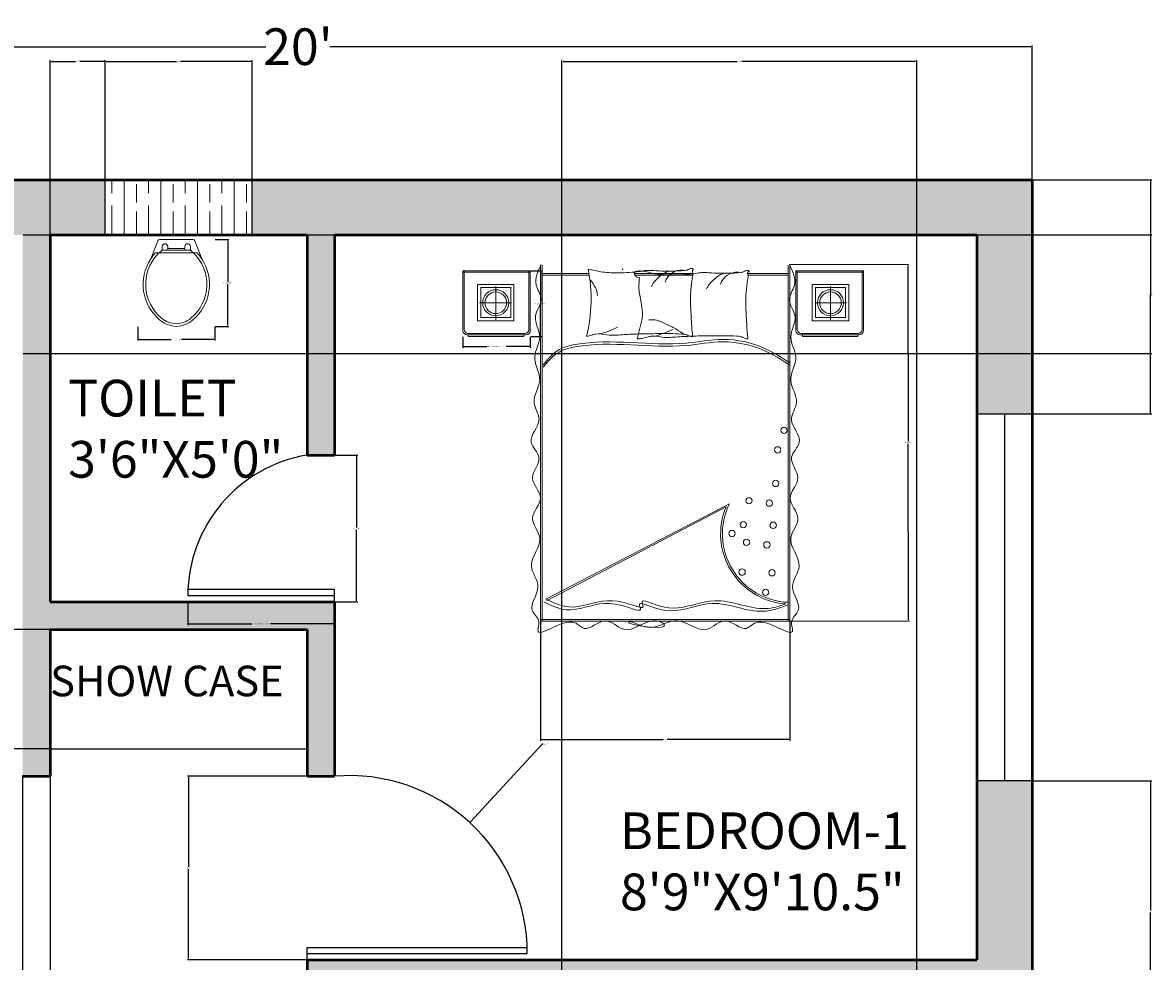
# Model space of a CAD drawing. Units: inches. Extents: x -2 to 282, y -370 to 35.
# Tile 5 of 5: x 97 to 282, y -119 to 35. Entities that reach past the tile are written whole.
import ezdxf

# ---------------------------------------------------------------- set-up
doc = ezdxf.new("R2010")
doc.units = ezdxf.units.IN
doc.header["$MEASUREMENT"] = 0
for name, color, linetype, lineweight in [('A-ANNO-DIMS', 2, 'Continuous', 18), ('A-ANNO-TEXT', 7, 'Continuous', 18), ('A-AREA-IDEN', 7, 'Continuous', 25), ('A-DOOR', 3, 'Continuous', 25), ('A-FLOR-CASE', 8, 'Continuous', 25), ('A-FLOR-FIXT', 9, 'Continuous', 18), ('A-FURN', 8, 'Continuous', 18), ('A-GLAZ', 4, 'Continuous', 25), ('A-GLAZ-PATT', 9, 'Continuous', 13), ('A-WALL', 7, 'Continuous', 50), ('A-WALL-PATT', 252, 'Continuous', 13)]:
    doc.layers.add(name, color=color, linetype=linetype, lineweight=lineweight)
doc.styles.get("Standard").update_dxf_attribs({"font": 'arial.ttf'})
doc.dimstyles.get("Standard").update_dxf_attribs({"dimtxt": 0.18, "dimasz": 0.18, "dimexe": 0.18, "dimexo": 0.0625, "dimgap": 0.09, "dimtad": 0, "dimtih": 1, "dimtoh": 1, "dimdec": 0, "dimzin": 0, "dimdsep": 46, "dimlunit": 3, "dimtxsty": 'Standard', "dimcen": 0.09, "dimadec": 0, "dimazin": 0, "dimtfac": 1, "dimtdec": 0, "dimtofl": 0, "dimtmove": 0, "dimatfit": 3, "dimfxl": 1, "dimtolj": 1, "dimtzin": 0, "dimarcsym": 0})

# ---------------------------------------------------------------- blocks, each defined once
blk = doc.blocks.new('*D3')
at = {"layer": 'A-ANNO-DIMS', "color": 0, "lineweight": -2, "transparency": 16777216}
for p, q in [((22.41, 9.25), (22.41, 31.14)), ((22.59, 30.96), (137.18, 30.96)), ((262.23, 30.96), (147.65, 30.96)), ((262.41, 9.25), (262.41, 31.14))]:
    blk.add_line(p, q, dxfattribs=at)
at = {"layer": 'A-ANNO-DIMS', "color": 0, "transparency": 16777216}
for points in [[(22.59, 30.99), (22.59, 30.93), (22.41, 30.96)], [(262.23, 30.99), (262.23, 30.93), (262.41, 30.96)]]:
    blk.add_solid(points, dxfattribs=at)
at = {"layer": 'Defpoints', "color": 0, "transparency": 16777216}
for p in [(262.41, 30.96), (22.41, 9.19), (262.41, 9.19)]:
    blk.add_point(p, dxfattribs=at)
at = {"layer": 'A-ANNO-DIMS', "color": 0, "transparency": 16777216, "insert": (142.41, 30.96), "char_height": 6, "attachment_point": 5}
blk.add_mtext("\\A1;20'", dxfattribs=at)
blk = doc.blocks.new('WINDOW-60IN')
for p, q in [((0, 0), (0, 60)), ((0, 60), (9, 60)), ((4.5, 60), (4.5, 0)), ((9, 60), (9, 0)), ((9, 0), (0, 0))]:
    blk.add_line(p, q)
blk = doc.blocks.new('DOOR-SWING-24IN')
for p, q in [((24, 2), (0, 2)), ((24, 0), (24, 2)), ((24, 1), (0, 1))]:
    blk.add_line(p, q)
blk.add_arc((23.32, 1), 23.31, 99.4157, 180)
blk = doc.blocks.new('WC-PLAN')
for p, q in [((2.03, 12.04), (2.63, 12.04)), ((2.63, 12.04), (5.42, 12.04)), ((8.21, 12.04), (5.42, 12.04)), ((8.21, 12.04), (8.81, 12.04))]:
    blk.add_line(p, q)
for points in [[(5.42, 14.19), (2.71, 14.19, 0.31031), (2.38, 13.97), (1.26, 11.07, 0.209071)], [(3.12, 12.47), (3.12, 13.07, -1), (4.02, 13.07), (4.02, 12.76)], [(5.42, 14.19), (8.13, 14.19, -0.31031), (8.46, 13.97), (9.58, 11.07, -0.209071)], [(7.72, 12.47), (7.72, 13.07, 1), (6.82, 13.07), (6.82, 12.76)], [(2.34, 11.76, 0.431639), (3.02, 1.35, 0.162618), (5.42, 0.42, 0.470877)], [(2.03, 12.04, 0.040937), (1.26, 11.07, 0.163732)], [(2.63, 12.04, 0.014165), (2.34, 11.76, 0.162618)], [(3.12, 12.47, 0.022712), (2.63, 12.04, 0.162618)], [(5.42, 12.47), (3.12, 12.47, 0.022712)], [(5.42, 12.47), (7.72, 12.47, -0.476108)], [(8.21, 12.04, -0.448546), (7.82, 1.35, -0.162618), (5.42, 0.42, -0.470877)], [(7.72, 12.47, -0.022712), (8.21, 12.04, -0.162618)], [(8.81, 12.04, -0.040937), (9.58, 11.07, -0.163732)], [(1.26, 11.07, 0.383919), (2.75, 1.02, 0.163732), (5.42, 0, 0.359733)], [(9.58, 11.07, -0.383919), (8.09, 1.02, -0.163732), (5.42, 0, -0.359733)]]:
    blk.add_lwpolyline(points, format="xyb")
for points in [[(6.82, 12.76), (4.02, 12.76)], [(4.02, 12.76), (4.02, 12.47)], [(6.82, 12.76), (6.82, 12.47)]]:
    blk.add_lwpolyline(points)
blk = doc.blocks.new('BEDSIDE-TABLE')
for p, q in [((0, 0.94), (0, 10.72)), ((0, 10.72), (11.02, 10.72)), ((0, 10.5), (11.02, 10.5)), ((0.22, 1.16), (0.22, 10.72)), ((10.8, 10.72), (10.8, 1.16)), ((11.02, 10.72), (11.02, 0.94)), ((2.39, 8.51), (2.39, 2.55)), ((8.35, 8.51), (2.39, 8.51)), ((2.92, 7.98), (2.92, 3.08)), ((7.82, 7.98), (2.92, 7.98)), ((5.37, 2.73), (5.37, 8.22)), ((7.82, 7.98), (7.82, 3.08)), ((8.35, 8.51), (8.35, 2.55)), ((7.94, 5.51), (2.73, 5.51)), ((8.35, 2.55), (2.39, 2.55)), ((7.82, 3.08), (2.92, 3.08)), ((10.37, 0.28), (0.66, 0.28)), ((10.15, 0.5), (0.87, 0.5))]:
    blk.add_line(p, q)
blk.add_lwpolyline([(9.94, 0.26), (0.88, 0.26), (0.88, 0), (9.94, 0)], close=True)
for radius in [2.13, 1.77]:
    blk.add_circle((5.37, 5.51), radius)
for centre, start, end in [((0.66, 0.94), 180, 270), ((0.87, 1.16), 180, 270), ((10.15, 1.16), 270, 0), ((10.37, 0.94), 270, 0)]:
    blk.add_arc(centre, 0.655, start, end)
blk = doc.blocks.new('*D13')
at = {"layer": 'A-ANNO-DIMS', "color": 0, "lineweight": -2, "transparency": 16777216}
for p, q in [((169.38, -16.48), (169.38, -18.25)), ((180.4, -16.48), (180.4, -18.25)), ((169.56, -18.07), (173.34, -18.07)), ((180.22, -18.07), (176.45, -18.07))]:
    blk.add_line(p, q, dxfattribs=at)
at = {"layer": 'A-ANNO-DIMS', "color": 0, "transparency": 16777216}
for points in [[(169.56, -18.04), (169.56, -18.1), (169.38, -18.07)], [(180.22, -18.04), (180.22, -18.1), (180.4, -18.07)]]:
    blk.add_solid(points, dxfattribs=at)
at = {"layer": 'Defpoints', "color": 0, "transparency": 16777216}
for p in [(169.38, -16.41), (180.4, -16.41), (180.4, -18.07)]:
    blk.add_point(p, dxfattribs=at)
at = {"layer": 'A-ANNO-DIMS', "color": 0, "transparency": 16777216, "insert": (174.89, -18.07), "char_height": 0.18, "attachment_point": 5}
blk.add_mtext('\\A1;NIGHTSTAND 0\'-11" TYP.', dxfattribs=at)
blk = doc.blocks.new('*D14')
at = {"layer": 'A-ANNO-DIMS', "color": 0, "lineweight": -2, "transparency": 16777216}
for p, q in [((180.46, -5.69), (182.24, -5.69)), ((182.06, -5.87), (182.06, -10.87)), ((182.06, -16.23), (182.06, -11.23)), ((180.46, -16.41), (182.24, -16.41))]:
    blk.add_line(p, q, dxfattribs=at)
at = {"layer": 'A-ANNO-DIMS', "color": 0, "transparency": 16777216}
for points in [[(182.03, -5.87), (182.09, -5.87), (182.06, -5.69)], [(182.03, -16.23), (182.09, -16.23), (182.06, -16.41)]]:
    blk.add_solid(points, dxfattribs=at)
at = {"layer": 'Defpoints', "color": 0, "transparency": 16777216}
for p in [(180.4, -5.69), (182.06, -5.69), (180.4, -16.41)]:
    blk.add_point(p, dxfattribs=at)
at = {"layer": 'A-ANNO-DIMS', "color": 0, "transparency": 16777216, "insert": (182.06, -11.05), "char_height": 0.18, "attachment_point": 5}
blk.add_mtext('\\A1;0\'-10 1/2" TYP.', dxfattribs=at)
blk = doc.blocks.new('*D17')
at = {"layer": 'A-ANNO-DIMS', "color": 0, "lineweight": -2, "transparency": 16777216}
for p, q in [((124.41, -59.87), (124.41, -63.59)), ((148.41, -59.87), (148.41, -63.59)), ((124.59, -63.41), (134.89, -63.41)), ((148.23, -63.41), (137.94, -63.41))]:
    blk.add_line(p, q, dxfattribs=at)
at = {"layer": 'A-ANNO-DIMS', "color": 0, "transparency": 16777216}
for points in [[(124.59, -63.38), (124.59, -63.44), (124.41, -63.41)], [(148.23, -63.38), (148.23, -63.44), (148.41, -63.41)]]:
    blk.add_solid(points, dxfattribs=at)
at = {"layer": 'Defpoints', "color": 0, "transparency": 16777216}
for p in [(124.41, -59.81), (148.41, -59.81), (148.41, -63.41)]:
    blk.add_point(p, dxfattribs=at)
at = {"layer": 'A-ANNO-DIMS', "color": 0, "transparency": 16777216, "insert": (136.41, -63.41), "char_height": 0.18, "attachment_point": 5}
blk.add_mtext('\\A1;TOILET DOOR 2\'-0" TYP.', dxfattribs=at)
blk = doc.blocks.new('*D18')
at = {"layer": 'A-ANNO-DIMS', "color": 0, "lineweight": -2, "transparency": 16777216}
for p, q in [((148.48, -35.81), (152.19, -35.81)), ((152.01, -35.99), (152.01, -47.63)), ((152.01, -59.63), (152.01, -47.99)), ((148.48, -59.81), (152.19, -59.81))]:
    blk.add_line(p, q, dxfattribs=at)
at = {"layer": 'A-ANNO-DIMS', "color": 0, "transparency": 16777216}
for points in [[(151.98, -35.99), (152.04, -35.99), (152.01, -35.81)], [(151.98, -59.63), (152.04, -59.63), (152.01, -59.81)]]:
    blk.add_solid(points, dxfattribs=at)
at = {"layer": 'Defpoints', "color": 0, "transparency": 16777216}
for p in [(148.41, -35.81), (152.01, -35.81), (148.41, -59.81)]:
    blk.add_point(p, dxfattribs=at)
at = {"layer": 'A-ANNO-DIMS', "color": 0, "transparency": 16777216, "insert": (152.01, -47.81), "char_height": 0.18, "attachment_point": 5}
blk.add_mtext('\\A1;2\'-0" TYP.', dxfattribs=at)
blk = doc.blocks.new('*D19')
at = {"layer": 'A-ANNO-DIMS', "color": 0, "lineweight": -2, "transparency": 16777216}
for p, q in [((128.9, -0.58), (131.14, -0.58)), ((130.96, -0.76), (130.96, -7.49)), ((130.96, -14.59), (130.96, -7.86)), ((128.9, -14.77), (131.14, -14.77))]:
    blk.add_line(p, q, dxfattribs=at)
at = {"layer": 'A-ANNO-DIMS', "color": 0, "transparency": 16777216}
for points in [[(130.93, -0.76), (130.99, -0.76), (130.96, -0.58)], [(130.93, -14.59), (130.99, -14.59), (130.96, -14.77)]]:
    blk.add_solid(points, dxfattribs=at)
at = {"layer": 'Defpoints', "color": 0, "transparency": 16777216}
for p in [(128.84, -0.58), (130.96, -0.58), (128.84, -14.77)]:
    blk.add_point(p, dxfattribs=at)
at = {"layer": 'A-ANNO-DIMS', "color": 0, "transparency": 16777216, "insert": (130.96, -7.67), "char_height": 0.18, "attachment_point": 5}
blk.add_mtext('\\A1;WC 1\'-2" TYP.', dxfattribs=at)
blk = doc.blocks.new('*D20')
at = {"layer": 'A-ANNO-DIMS', "color": 0, "lineweight": -2, "transparency": 16777216}
for p, q in [((116.23, -14.83), (116.23, -17.08)), ((128.84, -14.83), (128.84, -17.08)), ((116.41, -16.9), (121.69, -16.9)), ((128.66, -16.9), (123.37, -16.9))]:
    blk.add_line(p, q, dxfattribs=at)
at = {"layer": 'A-ANNO-DIMS', "color": 0, "transparency": 16777216}
for points in [[(116.41, -16.87), (116.41, -16.93), (116.23, -16.9)], [(128.66, -16.87), (128.66, -16.93), (128.84, -16.9)]]:
    blk.add_solid(points, dxfattribs=at)
at = {"layer": 'Defpoints', "color": 0, "transparency": 16777216}
for p in [(116.23, -14.77), (128.84, -14.77), (128.84, -16.9)]:
    blk.add_point(p, dxfattribs=at)
at = {"layer": 'A-ANNO-DIMS', "color": 0, "transparency": 16777216, "insert": (122.53, -16.9), "char_height": 0.18, "attachment_point": 5}
blk.add_mtext('\\A1;1\'-0 1/2" TYP.', dxfattribs=at)
blk = doc.blocks.new('*D25')
at = {"layer": 'A-ANNO-DIMS', "color": 0, "lineweight": -2, "transparency": 16777216}
for p, q in [((262.48, 9.19), (281.97, 9.19)), ((281.79, 9.01), (281.79, -9.75)), ((281.79, -28.88), (281.79, -10.12)), ((262.48, -29.06), (281.97, -29.06))]:
    blk.add_line(p, q, dxfattribs=at)
at = {"layer": 'A-ANNO-DIMS', "color": 0, "transparency": 16777216}
for points in [[(281.76, 9.01), (281.82, 9.01), (281.79, 9.19)], [(281.76, -28.88), (281.82, -28.88), (281.79, -29.06)]]:
    blk.add_solid(points, dxfattribs=at)
at = {"layer": 'Defpoints', "color": 0, "transparency": 16777216}
for p in [(262.41, 9.19), (262.41, -29.06), (281.79, -29.06)]:
    blk.add_point(p, dxfattribs=at)
at = {"layer": 'A-ANNO-DIMS', "color": 0, "transparency": 16777216, "insert": (281.79, -9.94), "char_height": 0.18, "attachment_point": 5}
blk.add_mtext('\\A1;3\'-2 1/2"', dxfattribs=at)
blk = doc.blocks.new('*D26')
at = {"layer": 'A-ANNO-DIMS', "color": 0, "lineweight": -2, "transparency": 16777216}
for p, q in [((262.48, -89.06), (281.97, -89.06)), ((281.79, -89.24), (281.79, -110.25)), ((281.79, -131.63), (281.79, -110.62)), ((262.48, -131.81), (281.97, -131.81))]:
    blk.add_line(p, q, dxfattribs=at)
at = {"layer": 'A-ANNO-DIMS', "color": 0, "transparency": 16777216}
for points in [[(281.76, -89.24), (281.82, -89.24), (281.79, -89.06)], [(281.76, -131.63), (281.82, -131.63), (281.79, -131.81)]]:
    blk.add_solid(points, dxfattribs=at)
at = {"layer": 'Defpoints', "color": 0, "transparency": 16777216}
for p in [(262.41, -89.06), (262.41, -131.81), (281.79, -131.81)]:
    blk.add_point(p, dxfattribs=at)
at = {"layer": 'A-ANNO-DIMS', "color": 0, "transparency": 16777216, "insert": (281.79, -110.44), "char_height": 0.18, "attachment_point": 5}
blk.add_mtext('\\A1;3\'-7"', dxfattribs=at)
blk = doc.blocks.new('*D33')
at = {"layer": 'A-ANNO-DIMS', "color": 0, "lineweight": -2, "transparency": 16777216}
for p, q in [((101.91, 0.25), (101.91, 28.74)), ((102.09, 28.56), (106.08, 28.56)), ((110.73, 28.56), (106.74, 28.56)), ((110.91, 0.25), (110.91, 28.74))]:
    blk.add_line(p, q, dxfattribs=at)
at = {"layer": 'A-ANNO-DIMS', "color": 0, "transparency": 16777216}
for points in [[(102.09, 28.59), (102.09, 28.53), (101.91, 28.56)], [(110.73, 28.59), (110.73, 28.53), (110.91, 28.56)]]:
    blk.add_solid(points, dxfattribs=at)
at = {"layer": 'Defpoints', "color": 0, "transparency": 16777216}
for p in [(110.91, 28.56), (101.91, 0.19), (110.91, 0.19)]:
    blk.add_point(p, dxfattribs=at)
at = {"layer": 'A-ANNO-DIMS', "color": 0, "transparency": 16777216, "insert": (106.41, 28.56), "char_height": 0.18, "attachment_point": 5}
blk.add_mtext('\\A1;0\'-9"', dxfattribs=at)
blk = doc.blocks.new('*D34')
at = {"layer": 'A-ANNO-DIMS', "color": 0, "lineweight": -2, "transparency": 16777216}
for p, q in [((110.91, 0.25), (110.91, 28.74)), ((111.09, 28.56), (122.58, 28.56)), ((134.73, 28.56), (123.24, 28.56)), ((134.91, 0.25), (134.91, 28.74))]:
    blk.add_line(p, q, dxfattribs=at)
at = {"layer": 'A-ANNO-DIMS', "color": 0, "transparency": 16777216}
for points in [[(111.09, 28.59), (111.09, 28.53), (110.91, 28.56)], [(134.73, 28.59), (134.73, 28.53), (134.91, 28.56)]]:
    blk.add_solid(points, dxfattribs=at)
at = {"layer": 'Defpoints', "color": 0, "transparency": 16777216}
for p in [(134.91, 28.56), (110.91, 0.19), (134.91, 0.19)]:
    blk.add_point(p, dxfattribs=at)
at = {"layer": 'A-ANNO-DIMS', "color": 0, "transparency": 16777216, "insert": (122.91, 28.56), "char_height": 0.18, "attachment_point": 5}
blk.add_mtext('\\A1;2\'-0"', dxfattribs=at)
blk = doc.blocks.new('*D39')
at = {"layer": 'A-ANNO-DIMS', "color": 0, "lineweight": -2, "transparency": 16777216}
for p, q in [((64.41, -88.37), (64.41, -370.37)), ((97.41, -88.37), (97.41, -370.37)), ((64.59, -370.19), (80.58, -370.19)), ((97.23, -370.19), (81.24, -370.19))]:
    blk.add_line(p, q, dxfattribs=at)
at = {"layer": 'A-ANNO-DIMS', "color": 0, "transparency": 16777216}
for points in [[(64.59, -370.16), (64.59, -370.22), (64.41, -370.19)], [(97.23, -370.16), (97.23, -370.22), (97.41, -370.19)]]:
    blk.add_solid(points, dxfattribs=at)
at = {"layer": 'Defpoints', "color": 0, "transparency": 16777216}
for p in [(64.41, -88.31), (97.41, -88.31), (97.41, -370.19)]:
    blk.add_point(p, dxfattribs=at)
at = {"layer": 'A-ANNO-DIMS', "color": 0, "transparency": 16777216, "insert": (80.91, -370.19), "char_height": 0.18, "attachment_point": 5}
blk.add_mtext('\\A1;2\'-9"', dxfattribs=at)
blk = doc.blocks.new('*D43')
at = {"layer": 'A-ANNO-DIMS', "color": 0, "lineweight": -2, "transparency": 16777216}
for p, q in [((97.48, 0.19), (281.97, 0.19)), ((281.79, 0.01), (281.79, -9.33)), ((281.79, -19.03), (281.79, -9.69)), ((97.48, -19.21), (281.97, -19.21))]:
    blk.add_line(p, q, dxfattribs=at)
at = {"layer": 'A-ANNO-DIMS', "color": 0, "transparency": 16777216}
for points in [[(281.76, 0.01), (281.82, 0.01), (281.79, 0.19)], [(281.76, -19.03), (281.82, -19.03), (281.79, -19.21)]]:
    blk.add_solid(points, dxfattribs=at)
at = {"layer": 'Defpoints', "color": 0, "transparency": 16777216}
for p in [(97.41, 0.19), (97.41, -19.21), (281.79, -19.21)]:
    blk.add_point(p, dxfattribs=at)
at = {"layer": 'A-ANNO-DIMS', "color": 0, "transparency": 16777216, "insert": (281.79, -9.51), "char_height": 0.18, "attachment_point": 5}
blk.add_mtext('\\A1;1\'-7 1/2"', dxfattribs=at)
blk = doc.blocks.new('*D45')
at = {"layer": 'A-ANNO-DIMS', "color": 0, "lineweight": -2, "transparency": 16777216}
for p, q in [((101.85, -64.31), (2.86, -64.31)), ((3.04, -64.49), (3.04, -73.88)), ((3.04, -83.63), (3.04, -74.24)), ((101.85, -83.81), (2.86, -83.81))]:
    blk.add_line(p, q, dxfattribs=at)
at = {"layer": 'A-ANNO-DIMS', "color": 0, "transparency": 16777216}
for points in [[(3.01, -64.49), (3.07, -64.49), (3.04, -64.31)], [(3.01, -83.63), (3.07, -83.63), (3.04, -83.81)]]:
    blk.add_solid(points, dxfattribs=at)
at = {"layer": 'Defpoints', "color": 0, "transparency": 16777216}
for p in [(101.91, -64.31), (3.04, -83.81), (101.91, -83.81)]:
    blk.add_point(p, dxfattribs=at)
at = {"layer": 'A-ANNO-DIMS', "color": 0, "transparency": 16777216, "insert": (3.04, -74.06), "char_height": 0.18, "attachment_point": 5}
blk.add_mtext('\\A1;1\'-7 1/2"', dxfattribs=at)
blk = doc.blocks.new('*D46')
at = {"layer": 'A-ANNO-DIMS', "color": 0, "lineweight": -2, "transparency": 16777216}
for p, q in [((97.41, -88.37), (97.41, -370.37)), ((101.91, -88.37), (101.91, -370.37)), ((97.59, -370.19), (99.12, -370.19)), ((101.73, -370.19), (100.2, -370.19))]:
    blk.add_line(p, q, dxfattribs=at)
at = {"layer": 'A-ANNO-DIMS', "color": 0, "transparency": 16777216}
for points in [[(97.59, -370.16), (97.59, -370.22), (97.41, -370.19)], [(101.73, -370.16), (101.73, -370.22), (101.91, -370.19)]]:
    blk.add_solid(points, dxfattribs=at)
at = {"layer": 'Defpoints', "color": 0, "transparency": 16777216}
for p in [(97.41, -88.31), (101.91, -88.31), (101.91, -370.19)]:
    blk.add_point(p, dxfattribs=at)
at = {"layer": 'A-ANNO-DIMS', "color": 0, "transparency": 16777216, "insert": (99.66, -370.19), "char_height": 0.18, "attachment_point": 5}
blk.add_mtext('\\A1;0\'-4 1/2"', dxfattribs=at)
blk = doc.blocks.new('*D52')
at = {"layer": 'A-ANNO-DIMS', "color": 0, "lineweight": -2, "transparency": 16777216}
for p, q in [((185.58, -222.52), (185.58, 28.74)), ((185.76, 28.56), (214.16, 28.56)), ((243.38, 28.56), (214.97, 28.56)), ((243.56, -222.52), (243.56, 28.74))]:
    blk.add_line(p, q, dxfattribs=at)
at = {"layer": 'A-ANNO-DIMS', "color": 0, "transparency": 16777216}
for points in [[(185.76, 28.59), (185.76, 28.53), (185.58, 28.56)], [(243.38, 28.59), (243.38, 28.53), (243.56, 28.56)]]:
    blk.add_solid(points, dxfattribs=at)
at = {"layer": 'Defpoints', "color": 0, "transparency": 16777216}
for p in [(243.56, 28.56), (185.58, -222.58), (243.56, -222.58)]:
    blk.add_point(p, dxfattribs=at)
at = {"layer": 'A-ANNO-DIMS', "color": 0, "transparency": 16777216, "insert": (214.57, 28.56), "char_height": 0.18, "attachment_point": 5}
blk.add_mtext('\\A1;4\'-10"', dxfattribs=at)
blk = doc.blocks.new('*D54')
at = {"layer": 'A-ANNO-DIMS', "color": 0, "lineweight": -2, "transparency": 16777216}
for p, q in [((182.07, -63.02), (182.07, -82.51)), ((222.85, -63.02), (222.85, -82.51)), ((182.25, -82.33), (202.13, -82.33)), ((222.67, -82.33), (202.79, -82.33))]:
    blk.add_line(p, q, dxfattribs=at)
at = {"layer": 'A-ANNO-DIMS', "color": 0, "transparency": 16777216}
for points in [[(182.25, -82.3), (182.25, -82.36), (182.07, -82.33)], [(222.67, -82.3), (222.67, -82.36), (222.85, -82.33)]]:
    blk.add_solid(points, dxfattribs=at)
at = {"layer": 'Defpoints', "color": 0, "transparency": 16777216}
for p in [(182.07, -62.96), (222.85, -62.96), (182.07, -82.33)]:
    blk.add_point(p, dxfattribs=at)
at = {"layer": 'A-ANNO-DIMS', "color": 0, "transparency": 16777216, "insert": (202.46, -82.33), "char_height": 0.18, "attachment_point": 5}
blk.add_mtext('\\A1;3\'-5"', dxfattribs=at)
blk = doc.blocks.new('*D55')
at = {"layer": 'A-ANNO-DIMS', "color": 0, "lineweight": -2, "transparency": 16777216}
for p, q in [((222.81, -4.64), (242.3, -4.61)), ((242.12, -4.79), (242.18, -33.58)), ((242.23, -62.74), (242.18, -33.95)), ((222.91, -62.96), (242.41, -62.92))]:
    blk.add_line(p, q, dxfattribs=at)
at = {"layer": 'A-ANNO-DIMS', "color": 0, "transparency": 16777216}
for points in [[(242.15, -4.79), (242.09, -4.79), (242.12, -4.61)], [(242.26, -62.74), (242.2, -62.74), (242.23, -62.92)]]:
    blk.add_solid(points, dxfattribs=at)
at = {"layer": 'Defpoints', "color": 0, "transparency": 16777216}
for p in [(222.75, -4.64), (222.85, -62.96), (242.23, -62.92)]:
    blk.add_point(p, dxfattribs=at)
at = {"layer": 'A-ANNO-DIMS', "color": 0, "transparency": 16777216, "insert": (242.18, -33.77), "char_height": 0.18, "attachment_point": 5}
blk.add_mtext('\\A1;4\'-10 1/2"', dxfattribs=at)
blk = doc.blocks.new('*D58')
at = {"layer": 'A-ANNO-DIMS', "color": 0, "lineweight": -2, "transparency": 16777216}
for p, q in [((143.85, -88.31), (124.36, -88.31)), ((124.54, -88.49), (124.54, -103.13)), ((124.54, -118.13), (124.54, -103.49)), ((143.85, -118.31), (124.36, -118.31))]:
    blk.add_line(p, q, dxfattribs=at)
at = {"layer": 'A-ANNO-DIMS', "color": 0, "transparency": 16777216}
for points in [[(124.51, -88.49), (124.57, -88.49), (124.54, -88.31)], [(124.51, -118.13), (124.57, -118.13), (124.54, -118.31)]]:
    blk.add_solid(points, dxfattribs=at)
at = {"layer": 'Defpoints', "color": 0, "transparency": 16777216}
for p in [(124.54, -88.31), (143.91, -88.31), (143.91, -118.31)]:
    blk.add_point(p, dxfattribs=at)
at = {"layer": 'A-ANNO-DIMS', "color": 0, "transparency": 16777216, "insert": (124.54, -103.31), "char_height": 0.18, "attachment_point": 5}
blk.add_mtext('\\A1;2\'-6"', dxfattribs=at)
blk = doc.blocks.new('*D60')
at = {"layer": 'A-ANNO-DIMS', "color": 0, "lineweight": -2, "transparency": 16777216}
for p, q in [((182.35, -83.06), (170.65, -95.77)), ((182.53, -83.06), (182.35, -83.06)), ((150.72, -117.31), (150.9, -117.31)), ((150.81, -117.4), (150.81, -117.22))]:
    blk.add_line(p, q, dxfattribs=at)
at = {"layer": 'A-ANNO-DIMS', "color": 0, "transparency": 16777216}
blk.add_solid([(170.62, -95.75), (170.67, -95.79), (170.52, -95.9)], dxfattribs=at)
at = {"layer": 'Defpoints', "color": 0, "transparency": 16777216}
for p in [(170.52, -95.9), (150.81, -117.31)]:
    blk.add_point(p, dxfattribs=at)
at = {"layer": 'A-ANNO-DIMS', "color": 0, "transparency": 16777216, "insert": (182.94, -83.06), "char_height": 0.18, "attachment_point": 5}
blk.add_mtext('\\A1;R2\'-5"', dxfattribs=at)

msp = doc.modelspace()

# ---------------------------------------------------------------- hatches: boundary and pattern name
at = {"layer": 'A-GLAZ-PATT'}
h = msp.add_hatch(dxfattribs=at)
h.set_pattern_fill('GOST_WOOD', color=256)
h.set_pattern_definition([(90, (0, 0), (6, -4e-16), [10, -2]), (90, (2, -2), (6, -4e-16), [6, -1.5, 3, -1.5]), (90, (4, -5), (6, -4e-16), [10, -2])])
h.paths.add_polyline_path([(134.91, 9.19), (110.91, 9.19), (110.91, 0.19), (134.91, 0.19)])
h.paths.add_polyline_path([(262.41, -131.81), (253.41, -131.81), (253.41, -155.81), (262.41, -155.81)])
at = {"layer": 'A-WALL-PATT'}
h = msp.add_hatch(color=256, dxfattribs=at)
h.dxf.hatch_style = 1
h.paths.add_polyline_path([(262.41, 9.19), (134.91, 9.19), (134.91, 0.19), (143.91, 0.19), (143.91, -35.81), (148.41, -35.81), (148.41, 0.19), (253.41, 0.19), (253.41, -29.06), (262.41, -29.06)])
h.paths.add_polyline_path([(110.91, 9.19), (22.41, 9.19), (22.41, -11.81), (31.41, -11.81), (31.41, 0.19), (97.41, 0.19), (97.41, -88.31), (101.91, -88.31), (101.91, -64.31), (143.91, -64.31), (143.91, -88.31), (148.41, -88.31), (148.41, -59.81), (101.91, -59.81), (101.91, 0.19), (110.91, 0.19)])
h.paths.add_polyline_path([(31.41, -88.31), (64.41, -88.31), (64.41, -83.81), (31.41, -83.81), (31.41, -71.81), (22.41, -71.81), (22.41, -121.2), (31.41, -121.2)])
h.paths.add_polyline_path([(262.41, -89.06), (253.41, -89.06), (253.41, -118.31), (143.91, -118.31), (143.91, -122.81), (184.41, -122.81), (184.41, -164.81), (184.41, -169.31), (188.91, -169.31), (188.91, -164.81), (188.91, -122.81), (253.41, -122.81), (253.41, -131.81), (262.41, -131.81)])
h.paths.add_polyline_path([(262.41, -155.81), (253.41, -155.81), (253.41, -164.81), (212.91, -164.81), (212.91, -169.31), (253.41, -169.31), (253.41, -193.31), (262.41, -193.31)])
h.paths.add_polyline_path([(262.41, -253.31), (253.41, -253.31), (253.41, -277.31), (148.41, -277.31), (148.41, -164.81), (143.91, -164.81), (143.91, -169.31), (143.91, -281.81), (253.41, -281.81), (253.41, -341.81), (143.91, -341.81), (143.91, -350.81), (262.41, -350.81)])
h.paths.add_polyline_path([(31.41, -323.81), (22.41, -323.81), (22.41, -350.81), (95.91, -350.81), (95.91, -281.81), (107.91, -281.81), (107.91, -277.31), (67.41, -277.31), (67.41, -281.81), (91.41, -281.81), (91.41, -341.81), (31.41, -341.81)])
h.paths.add_polyline_path([(43.41, -277.31), (31.41, -277.31), (31.41, -181.2), (22.41, -181.2), (22.41, -299.81), (31.41, -299.81), (31.41, -281.81), (43.41, -281.81)])

# ---------------------------------------------------------------- linework, layer by layer
at = {"layer": 'A-DOOR'}
for p, q in [((143.91, -118.31), (143.91, -116.31)), ((143.91, -116.31), (179.91, -116.31)), ((143.91, -117.31), (179.91, -117.31))]:
    msp.add_line(p, q, dxfattribs=at)
msp.add_arc((150.81, -117.31), 29.1, 0, 94.7325, dxfattribs=at)
at = {"layer": 'A-FLOR-CASE'}
msp.add_line((101.91, -83.81), (143.91, -83.81), dxfattribs=at)
at = {"layer": 'A-FURN'}
for p, q in [((182.07, -4.74), (182.07, -62.96)), ((182.36, -4.74), (182.36, -62.96)), ((222.56, -4.74), (222.56, -62.96)), ((222.85, -4.74), (222.85, -62.96)), ((182.36, -6.13), (189.99, -6.13)), ((182.36, -6.42), (190.04, -6.42)), ((206.97, -6.13), (197.39, -6.13)), ((206.97, -6.42), (197.5, -6.42)), ((215.92, -6.13), (222.56, -6.13)), ((216, -6.42), (222.56, -6.42)), ((198.08, -15.91), (198.68, -13.51)), ((197.86, -16.79), (198.08, -15.91)), ((182.95, -59.35), (212.94, -43.77)), ((183.06, -59.63), (212.39, -44.28)), ((182.07, -62.67), (222.85, -62.67)), ((182.07, -62.96), (222.85, -62.96))]:
    msp.add_line(p, q, dxfattribs=at)
for centre in [(221.86, -31.75), (220.83, -34.96), (220.52, -40.45), (216.16, -43.25), (219.48, -43.66), (215.23, -47.18), (220.1, -47.28), (213.37, -48.63), (215.75, -50.08), (219.07, -50.49), (215.02, -54.95), (219.9, -55.05), (218.86, -58.26)]:
    msp.add_circle(centre, 0.518, dxfattribs=at)
for centre, radius, start, end in [((165.2, -10.28), 25.14, 345.9578, 11.1903), ((188.56, -14.18), 8.87, 74.256, 81.5628), ((195.46, -5.43), 0.0675, 258.1069, 19.564), ((195.43, -5.44), 0.0995, 19.564, 68.2117), ((205.57, -4.06), 1.57, 275.2592, 300.6513), ((206.8, -6.13), 0.841, 85.6975, 120.6513), ((206.81, -6.02), 0.731, 68.2117, 85.6975), ((207.03, -5.62), 0.125, 78.1069, 158.0096), ((187.34, -10.12), 4.07, 5.6311, 45.0976), ((192.88, 1.14), 7.05, 254.256, 262.4531), ((194.56, 13.85), 19.87, 262.4531, 270), ((194.56, 24.52), 30.53, 270, 276.0867), ((197.77, -6.13), 0.382, 101.2724, 206.5805), ((198.32, -5.85), 0.995, 206.5805, 265.5998), ((198.21, -8.33), 2.63, 90, 101.2724), ((196.17, 9.47), 15.41, 276.0867, 280.1899), ((212.47, -8.39), 14.32, 173.7676, 180), ((198.21, -10.39), 4.69, 81.5628, 90), ((199.68, -10.05), 4.44, 92.5386, 100.1899), ((197.6, -14.53), 8.87, 74.256, 81.5628), ((199.86, -14.05), 8.43, 85.1982, 92.5386), ((201.92, 0.8), 7.05, 254.256, 262.4531), ((202.69, 19.68), 25.42, 265.1982, 269.4243), ((205.67, -11.72), 6.55, 133.8115, 140.9651), ((203.6, 13.51), 19.87, 262.4531, 270), ((209.02, -15.21), 11.4, 128.3886, 133.8115), ((203.33, -8.03), 2.23, 117.2396, 128.3886), ((205.42, -12.1), 6.81, 110.8603, 117.2396), ((205.17, -8.45), 2.89, 85.7841, 161.5603), ((202.87, 37.76), 43.49, 269.4243, 271.9079), ((203.6, 24.17), 30.53, 270, 276.0867), ((203.52, 18.17), 23.89, 271.9079, 275.2592), ((233.14, -10.87), 26.58, 172.3191, 176.6313), ((212.53, -8.09), 5.77, 167.8905, 172.3191), ((205.2, 9.13), 15.41, 276.0867, 280.1899), ((207.34, -5.74), 0.454, 158.0096, 201.421), ((199.88, -5.38), 7.16, 347.8905, 351.8665), ((206.03, -6.25), 0.954, 351.8665, 21.421), ((208.71, -10.4), 4.44, 92.5386, 100.1899), ((208.89, -14.39), 8.43, 85.1982, 92.5386), ((211.72, 19.34), 25.42, 265.1982, 269.4243), ((214.7, -12.07), 6.55, 133.8115, 140.9651), ((218.06, -15.56), 11.4, 128.3886, 133.8115), ((212.36, -8.38), 2.23, 117.2396, 128.3886), ((214.46, -12.45), 6.81, 110.8603, 117.2396), ((214.21, -8.8), 2.89, 85.7841, 161.5603), ((211.91, 37.41), 43.49, 269.4243, 271.9079), ((212.56, 17.82), 23.89, 271.9079, 275.2592), ((214.6, -4.41), 1.57, 275.2592, 300.6513), ((215.83, -6.48), 0.841, 85.6975, 120.6513), ((221.56, -8.44), 5.77, 167.8905, 172.3191), ((215.84, -6.37), 0.731, 68.2117, 85.6975), ((216.37, -6.09), 0.454, 158.0096, 201.421), ((208.92, -5.72), 7.16, 347.8905, 351.8665), ((216.07, -5.96), 0.125, 78.1069, 158.0096), ((215.06, -6.6), 0.954, 351.8665, 21.421), ((216.11, -5.77), 0.0675, 258.1069, 19.564), ((216.08, -5.79), 0.0995, 19.564, 68.2117), ((204.09, -8.39), 5.94, 180, 189.6844), ((205.56, -10.58), 5.83, 151.6832, 156.9972), ((201.69, -8.49), 1.44, 140.9651, 151.6832), ((214.59, -10.92), 5.83, 151.6832, 156.9972), ((210.73, -8.84), 1.44, 140.9651, 151.6832), ((242.18, -11.22), 26.58, 172.3191, 176.6313), ((223.54, -5.07), 25.67, 189.6844, 192.1984), ((189.43, -12.45), 9.23, 8.0051, 12.1984), ((226.34, -10.47), 19.76, 176.6313, 181.6331), ((246.31, -9.9), 39.74, 181.6331, 183.055), ((235.37, -10.82), 19.76, 176.6313, 181.6331), ((179.58, -13.83), 19.18, 2.6649, 8.0051), ((602.96, 9.14), 396.89, 183.055, 183.5049), ((255.35, -10.25), 39.74, 181.6331, 183.055), ((611.99, 8.79), 396.89, 183.055, 183.5049), ((196.77, -13.03), 1.97, 345.9548, 2.6649), ((200.25, -21.61), 7.92, 85.9172, 93.5552), ((200.69, -15.4), 1.69, 69.3257, 85.9172), ((196.08, -27.61), 14.75, 65.6735, 69.3257), ((184.98, -52.17), 41.69, 63.5015, 65.6735), ((188.49, -9.79), 6.69, 279.4841, 287.3864), ((191.53, -19.5), 3.49, 96.4341, 107.3864), ((191.61, -20.25), 4.25, 78.4414, 96.4341), ((185.48, 4.53), 21.5, 287.1982, 295.3111), ((193.8, -9.53), 6.7, 258.4414, 272.7491), ((192.16, 24.62), 40.89, 272.7491, 274.6176), ((198.31, -51.43), 35.41, 92.6096, 94.6176), ((201.15, -113.82), 97.86, 90.9704, 92.6096), ((197.52, -10.14), 6.69, 279.4841, 287.3864), ((202.31, -182.4), 166.45, 89.7135, 90.9704), ((200.56, -19.84), 3.49, 96.4341, 107.3864), ((200.65, -20.6), 4.25, 78.4414, 96.4341), ((194.52, 4.18), 21.5, 287.1982, 295.3111), ((202.84, -9.88), 6.7, 258.4414, 272.7491), ((202.98, -49.83), 33.88, 86.426, 89.7135), ((201.2, 24.27), 40.89, 272.7491, 274.6176), ((199.52, -23), 9.1, 57.865, 63.5015), ((193.08, -33.25), 21.21, 54.1737, 57.865), ((207.34, -51.77), 35.41, 92.6096, 94.6176), ((204.82, -20.25), 4.25, 77.131, 86.426), ((210.19, -114.17), 97.86, 90.9704, 92.6096), ((205.47, -17.4), 1.32, 62.7159, 77.131), ((207.1, -14.24), 2.23, 242.7159, 253.7788), ((207.19, -13.94), 2.55, 253.7788, 262.8796), ((216.14, -14.56), 9.35, 183.5049, 189.9984), ((206.88, -16.43), 0.0385, 262.8796, 343.3022), ((206.38, -16.28), 0.563, 343.3022, 9.9984), ((211.35, -182.74), 166.45, 89.7135, 90.9704), ((212.01, -50.18), 33.88, 86.426, 89.7135), ((213.86, -20.6), 4.25, 77.131, 86.426), ((214.51, -17.74), 1.32, 62.7159, 77.131), ((216.14, -14.59), 2.23, 242.7159, 253.7788), ((225.17, -14.9), 9.35, 183.5049, 189.9984), ((215.41, -16.62), 0.563, 343.3022, 9.9984), ((197.88, -16.79), 0.0267, 165.9551, 274.0829), ((197.33, -8.96), 7.88, 274.0829, 279.4841), ((216.23, -14.29), 2.55, 253.7788, 262.8796), ((215.91, -16.77), 0.0385, 262.8796, 343.3022), ((223, -48.69), 11.49, 157.4442, 265.7493), ((223, -48.69), 11.2, 153.9063, 267.7674)]:
    msp.add_arc(centre, radius, start, end, dxfattribs=at)
for points, knots in [([(182.17, -4.64), (181.63, -5.78), (180.7, -7.72), (182.88, -10.49), (180.39, -13.27), (182.74, -16.5), (180.26, -19.94), (182.9, -23.55), (180.13, -26.96), (182.87, -30.32), (179.29, -33.44), (182.95, -36.33), (179.53, -39.58), (183.31, -42.82), (179.62, -46.1), (183.31, -49.76), (179.24, -53.61), (182.82, -57.4), (179.58, -60.87), (182.19, -62.65), (180.72, -66.65), (186.76, -61.48), (189.58, -65.14), (192.61, -61.59), (196.07, -65.77), (200.33, -61.51), (204.55, -64.87), (195.53, -63.31), (196.66, -63.02)], [0, 0, 0, 0, 119.23822, 203.934156, 305.051348, 423.414205, 538.771408, 673.601551, 801.564672, 901.488314, 1036.739405, 1131.503109, 1252.869042, 1373.114912, 1497.089457, 1612.174498, 1779.078494, 1901.133447, 2037.052147, 2110.507177, 2158.377997, 2368.992723, 2430.676444, 2554.510696, 2670.523569, 2841.287389, 2999.108306, 3118.80064, 3118.80064, 3118.80064, 3118.80064]), ([(222.75, -4.64), (223.29, -5.78), (224.22, -7.72), (222.04, -10.49), (224.53, -13.27), (222.18, -16.5), (224.66, -19.94), (222.02, -23.55), (224.79, -26.96), (222.05, -30.32), (225.63, -33.44), (221.96, -36.33), (225.38, -39.58), (221.61, -42.82), (225.3, -46.1), (221.61, -49.76), (225.68, -53.61), (222.1, -57.4), (225.34, -60.87), (222.73, -62.65), (224.2, -66.65), (218.16, -61.48), (215.34, -65.14), (212.31, -61.59), (208.85, -65.77), (204.59, -61.51), (200.37, -64.87), (197.78, -63.31), (196.66, -63.02)], [0, 0, 0, 0, 119.23822, 203.934156, 305.051348, 423.414205, 538.771408, 673.601551, 801.564672, 901.488314, 1036.739405, 1131.503109, 1252.869042, 1373.114912, 1497.089457, 1612.174498, 1779.078494, 1901.133447, 2037.052147, 2110.507177, 2158.377997, 2368.992723, 2430.676444, 2554.510696, 2670.523569, 2841.287389, 2999.108306, 3118.80064, 3118.80064, 3118.80064, 3118.80064]), ([(182.49, -21.06), (183.29, -20.11), (184.68, -18.42), (192.88, -16.42), (201.89, -18.52), (212.15, -16.46), (218.16, -17.74), (221.46, -19.84), (222.81, -20.71)], [0, 0, 0, 0, 3.612443, 6.355405, 24.536278, 30.541821, 37.462744, 42.251599, 42.251599, 42.251599, 42.251599]), ([(182.49, -21.45), (183.29, -20.49), (184.68, -18.81), (192.88, -16.81), (201.89, -18.91), (212.15, -16.85), (218.16, -18.12), (221.46, -20.23), (222.81, -21.09)], [0, 0, 0, 0, 3.612443, 6.355405, 24.536278, 30.541821, 37.462744, 42.251599, 42.251599, 42.251599, 42.251599]), ([(182.59, -59.81), (183.81, -60.4), (187, -61.94), (192.79, -58.97), (200.42, -62.56), (196.4, -58.85), (203.73, -62.27), (210.61, -58.72), (217.14, -62.24), (221.2, -60.8), (222.56, -60.29)], [0, 0, 0, 0, 134.096191, 351.943146, 593.51487, 936.925241, 1129.231545, 1368.385454, 1657.415202, 1803.02854, 1803.02854, 1803.02854, 1803.02854]), ([(183, -59.36), (184.22, -59.95), (187.42, -61.49), (193.21, -58.52), (200.83, -62.11), (196.82, -58.4), (204.14, -61.82), (211.03, -58.27), (217.27, -61.64), (221.06, -60.53), (222.15, -60.15)], [0, 0, 0, 0, 134.096191, 351.943146, 593.51487, 936.925241, 1129.231545, 1368.385454, 1657.415202, 1773.3935, 1773.3935, 1773.3935, 1773.3935])]:
    msp.add_open_spline(points, degree=3, knots=knots, dxfattribs=at)
at = {"layer": 'A-GLAZ'}
for p, q in [((110.91, 0.19), (110.91, 9.19)), ((134.91, 0.19), (134.91, 9.19))]:
    msp.add_line(p, q, dxfattribs=at)
at = {"layer": 'A-WALL'}
for p, q in [((22.41, 9.19), (262.41, 9.19)), ((262.41, 9.19), (262.41, -350.81)), ((101.91, 0.19), (101.91, -59.81)), ((101.91, 0.19), (143.91, 0.19)), ((143.91, 0.19), (143.91, -35.81)), ((148.41, 0.19), (148.41, -35.81)), ((148.41, 0.19), (253.41, 0.19)), ((253.41, 0.19), (253.41, -118.31)), ((143.91, -35.81), (148.41, -35.81)), ((101.91, -59.81), (148.41, -59.81)), ((148.41, -59.81), (148.41, -88.31)), ((101.91, -64.31), (143.91, -64.31)), ((101.91, -64.31), (101.91, -88.31)), ((143.91, -64.31), (143.91, -88.31)), ((97.41, -88.31), (101.91, -88.31)), ((143.91, -88.31), (148.41, -88.31)), ((143.91, -118.31), (253.41, -118.31)), ((143.91, -118.31), (143.91, -122.81))]:
    msp.add_line(p, q, dxfattribs=at)

# ---------------------------------------------------------------- block references
at = {"layer": 'A-DOOR'}
msp.add_blockref('DOOR-SWING-24IN', (124.41, -59.81), dxfattribs=at)
at = {"layer": 'A-FLOR-FIXT'}
msp.add_blockref('WC-PLAN', (117.11, -14.77), dxfattribs=at)
at = {"layer": 'A-FURN'}
msp.add_blockref('BEDSIDE-TABLE', (169.38, -16.41), dxfattribs=at)
at = {"layer": 'A-FURN', "extrusion": (0, 0, -1), "zscale": -1}
msp.add_blockref('BEDSIDE-TABLE', (-234.84, -16.41), dxfattribs=at)
at = {"layer": 'A-GLAZ'}
msp.add_blockref('WINDOW-60IN', (253.41, -89.06), dxfattribs=at)

# ---------------------------------------------------------------- texts
at = {"layer": 'A-ANNO-TEXT', "insert": (101.91, -70.24), "char_height": 5, "attachment_point": 1}
msp.add_mtext('SHOW CASE', dxfattribs=at)
at = {"layer": 'A-AREA-IDEN', "char_height": 6, "attachment_point": 1}
for s, insert in [('TOILET\\P3\'6"X5\'0"', (104.86, -23.5)), ('BEDROOM-1\\P8\'9"X9\'10.5"', (195.06, -94.23))]:
    msp.add_mtext(s, dxfattribs=dict(at, insert=insert))

# ---------------------------------------------------------------- dimensions: what is measured, and where the dimension line sits
at = {"layer": 'A-ANNO-DIMS'}
for base, p1, p2, override, picture, middle in [((262.41, 30.96), (22.41, 9.19), (262.41, 9.19), {"dimtxt": 6, "dimclrd": 0, "dimclre": 0, "dimclrt": 0}, '*D3', (142.41, 30.96)), ((110.91, 28.56), (101.91, 0.19), (110.91, 0.19), {"dimdec": 1, "dimlfac": 1, "dimrnd": 0, "dimzin": 1, "dimdsep": 46, "dimlunit": 4, "dimfrac": 2}, '*D33', (106.41, 28.56)), ((134.91, 28.56), (110.91, 0.19), (134.91, 0.19), {"dimdec": 1, "dimlfac": 1, "dimrnd": 0, "dimzin": 1, "dimdsep": 46, "dimlunit": 4, "dimfrac": 2}, '*D34', (122.91, 28.56)), ((243.56, 28.56), (185.58, -222.58), (243.56, -222.58), {"dimdec": 1, "dimlfac": 1, "dimrnd": 0, "dimzin": 1, "dimdsep": 46, "dimlunit": 4, "dimfrac": 2}, '*D52', (214.57, 28.56)), ((97.41, -370.19), (64.41, -88.31), (97.41, -88.31), {"dimdec": 1, "dimlfac": 1, "dimrnd": 0, "dimzin": 1, "dimdsep": 46, "dimlunit": 4, "dimfrac": 2}, '*D39', (80.91, -370.19)), ((101.91, -370.19), (97.41, -88.31), (101.91, -88.31), {"dimdec": 1, "dimlfac": 1, "dimrnd": 0, "dimzin": 1, "dimdsep": 46, "dimlunit": 4, "dimfrac": 2}, '*D46', (99.66, -370.19))]:
    dim = msp.add_linear_dim(base=base, p1=p1, p2=p2, dimstyle='Standard', override=override, dxfattribs=at)
    dim.commit()
    dim.dimension.update_dxf_attribs({"geometry": picture, "text_midpoint": middle})
for base, p1, p2, angle, picture, middle in [((281.788386, -29.0601), (262.413386, 9.1899), (262.413386, -29.0601), 90, '*D25', (281.788386, -9.9351)), ((281.79, -19.21), (97.41, 0.19), (97.41, -19.21), 90, '*D43', (281.79, -9.51)), ((242.23, -62.92), (222.75, -4.64), (222.85, -62.96), 270.1006, '*D55', (242.18, -33.77)), ((3.04, -83.81), (101.91, -64.31), (101.91, -83.81), 90, '*D45', (3.04, -74.06)), ((182.07, -82.33), (222.85, -62.96), (182.07, -62.96), 180, '*D54', (202.46, -82.33)), ((124.54, -88.31), (143.91, -118.31), (143.91, -88.31), 90, '*D58', (124.54, -103.31)), ((281.788386, -131.8101), (262.413386, -89.0601), (262.413386, -131.8101), 90, '*D26', (281.788386, -110.4351))]:
    dim = msp.add_linear_dim(base=base, p1=p1, p2=p2, angle=angle, dimstyle='Standard', override={"dimdec": 1, "dimlfac": 1, "dimrnd": 0, "dimzin": 1, "dimdsep": 46, "dimlunit": 4, "dimfrac": 2}, dxfattribs=at)
    dim.commit()
    dim.dimension.update_dxf_attribs({"geometry": picture, "text_midpoint": middle})
for base, p1, p2, text, picture, middle in [((130.96, -0.58), (128.84, -14.77), (128.84, -0.58), 'WC <> TYP.', '*D19', (130.96, -7.67)), ((182.06, -5.69), (180.4, -16.41), (180.4, -5.69), '<> TYP.', '*D14', (182.06, -11.05)), ((152.01, -35.81), (148.41, -59.81), (148.41, -35.81), '<> TYP.', '*D18', (152.01, -47.81))]:
    dim = msp.add_linear_dim(base=base, p1=p1, p2=p2, angle=90, text=text, dimstyle='Standard', override={"dimdec": 1, "dimlfac": 1, "dimrnd": 0, "dimzin": 1, "dimdsep": 46, "dimlunit": 4, "dimfrac": 2}, dxfattribs=at)
    dim.commit()
    dim.dimension.update_dxf_attribs({"geometry": picture, "text_midpoint": middle})
for base, p1, p2, text, picture, middle in [((128.84, -16.9), (116.23, -14.77), (128.84, -14.77), '<> TYP.', '*D20', (122.53, -16.9)), ((180.4, -18.07), (169.38, -16.41), (180.4, -16.41), 'NIGHTSTAND <> TYP.', '*D13', (174.89, -18.07)), ((148.41, -63.41), (124.41, -59.81), (148.41, -59.81), 'TOILET DOOR <> TYP.', '*D17', (136.41, -63.41))]:
    dim = msp.add_linear_dim(base=base, p1=p1, p2=p2, text=text, dimstyle='Standard', override={"dimdec": 1, "dimlfac": 1, "dimrnd": 0, "dimzin": 1, "dimdsep": 46, "dimlunit": 4, "dimfrac": 2}, dxfattribs=at)
    dim.commit()
    dim.dimension.update_dxf_attribs({"geometry": picture, "text_midpoint": middle})
dim = msp.add_radius_dim(center=(150.81, -117.31), mpoint=(170.52, -95.9), dimstyle='Standard', override={"dimdec": 1, "dimlfac": 1, "dimrnd": 0, "dimzin": 1, "dimdsep": 46, "dimlunit": 4, "dimfrac": 2}, dxfattribs=at)
dim.commit()
dim.dimension.update_dxf_attribs({"geometry": '*D60', "text_midpoint": (182.94, -83.06), "dimtype": 164})

doc.saveas('drawing.dxf')
